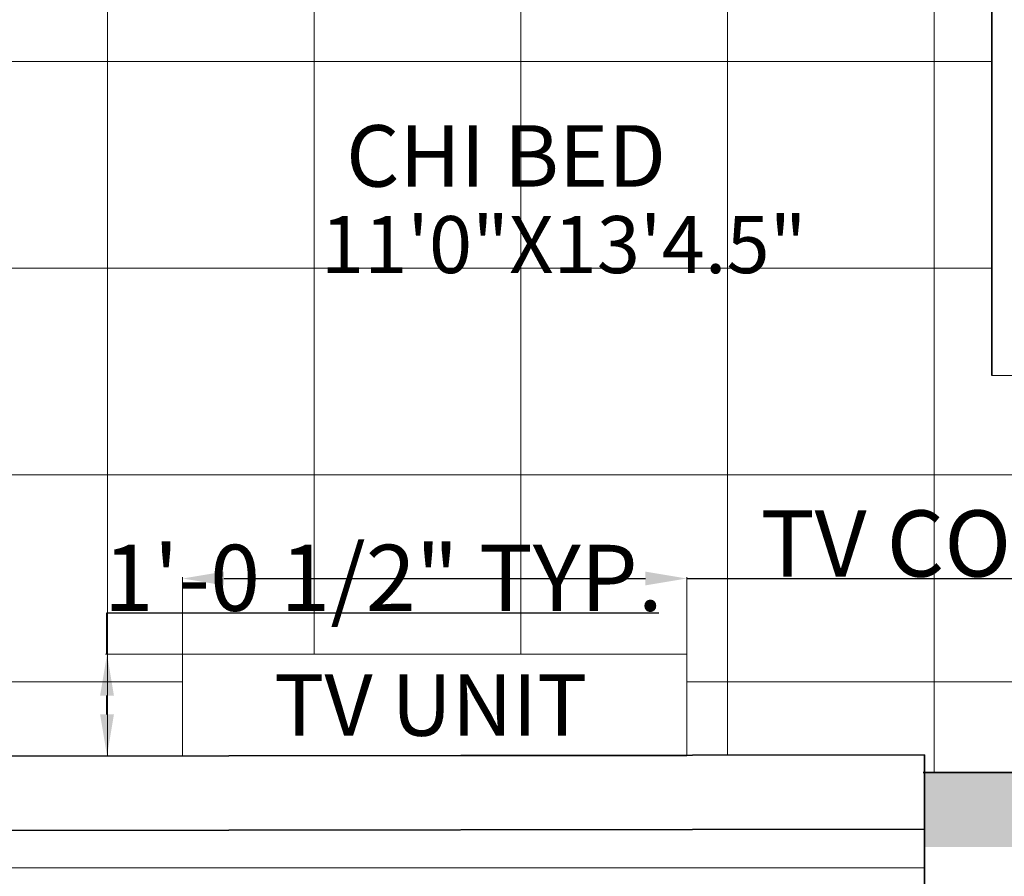
# Model space of a CAD drawing. Units: inches. Extents: x 351 to 1738, y -265 to 286.
# Tile 22 of 38: x 1127 to 1246, y -63 to 41. Entities that reach past the tile are written whole.
import ezdxf

# ---------------------------------------------------------------- set-up
doc = ezdxf.new("R2010")
doc.units = ezdxf.units.IN
doc.header["$MEASUREMENT"] = 0
for name, color, linetype, lineweight in [('A-ANNO-DIMS', 2, 'Continuous', 18), ('A-ANNO-TEXT', 7, 'Continuous', 18), ('A-AREA-IDEN', 7, 'Continuous', 18), ('A-COLS-PATT', 6, 'Continuous', 13), ('A-DOOR', 3, 'Continuous', 18), ('A-FLOR-CASE', 9, 'Continuous', 18), ('A-FLOR-PATT', 9, 'Continuous', 9), ('A-WALL', 7, 'Continuous', 35)]:
    doc.layers.add(name, color=color, linetype=linetype, lineweight=lineweight)
doc.styles.add('Annotative', font='arial.ttf')
doc.styles.get("Standard").update_dxf_attribs({"font": 'arial.ttf'})
doc.dimstyles.get("Standard").update_dxf_attribs({"dimtxt": 8, "dimasz": 5, "dimexe": 0.18, "dimexo": 0.0625, "dimgap": 0.09, "dimtad": 1, "dimtoh": 1, "dimzin": 0, "dimdsep": 46, "dimlunit": 4, "dimtxsty": 'Standard', "dimcen": 0, "dimclre": 256, "dimadec": 0, "dimazin": 0, "dimtfac": 1, "dimtofl": 0, "dimtmove": 0, "dimatfit": 3, "dimfxl": 1, "dimtolj": 1, "dimtzin": 0, "dimlwe": -1, "dimarcsym": 0})

# ---------------------------------------------------------------- blocks, each defined once
blk = doc.blocks.new('CONSOLE-TV')
blk.add_lwpolyline([(0, 0), (61, 0), (61, 12.29), (0, 12.29)], close=True)
blk = doc.blocks.new('*D42')
at = {"layer": 'A-ANNO-DIMS', "transparency": 16777216}
for p, q in [((1146.8, -35.63), (1146.8, -26.36)), ((1207.8, -35.63), (1207.8, -26.36))]:
    blk.add_line(p, q, dxfattribs=at)
at = {"layer": 'A-ANNO-DIMS', "color": 0, "lineweight": -2, "transparency": 16777216}
for p, q in [((1151.8, -26.54), (1202.8, -26.54)), ((1207.8, -26.54), (1337.09, -26.54))]:
    blk.add_line(p, q, dxfattribs=at)
at = {"layer": 'A-ANNO-DIMS', "color": 0, "transparency": 16777216}
for points in [[(1151.8, -25.71), (1151.8, -27.37), (1146.8, -26.54)], [(1202.8, -25.71), (1202.8, -27.37), (1207.8, -26.54)]]:
    blk.add_solid(points, dxfattribs=at)
at = {"layer": 'Defpoints', "color": 0, "transparency": 16777216}
for p in [(1207.8, -26.54), (1146.8, -35.69), (1207.8, -35.69)]:
    blk.add_point(p, dxfattribs=at)
at = {"layer": 'A-ANNO-DIMS', "color": 0, "transparency": 16777216, "insert": (1274.95, -22.31), "char_height": 8, "attachment_point": 5}
blk.add_mtext('\\A1;TV CONSOLE 5\'-1" TYP.', dxfattribs=at)
blk = doc.blocks.new('*D43')
at = {"layer": 'A-ANNO-DIMS', "color": 0, "lineweight": -2, "transparency": 16777216}
for p, q in [((1137.65, -35.69), (1137.65, -30.69)), ((1137.65, -30.69), (1204.4, -30.69)), ((1137.65, -42.98), (1137.65, -40.69))]:
    blk.add_line(p, q, dxfattribs=at)
at = {"layer": 'A-ANNO-DIMS', "transparency": 16777216}
for p, q in [((1146.74, -35.69), (1137.47, -35.69)), ((1146.74, -47.98), (1137.47, -47.98))]:
    blk.add_line(p, q, dxfattribs=at)
at = {"layer": 'A-ANNO-DIMS', "color": 0, "transparency": 16777216}
for points in [[(1136.82, -40.69), (1138.49, -40.69), (1137.65, -35.69)], [(1136.82, -42.98), (1138.49, -42.98), (1137.65, -47.98)]]:
    blk.add_solid(points, dxfattribs=at)
at = {"layer": 'Defpoints', "color": 0, "transparency": 16777216}
for p in [(1137.65, -35.69), (1146.8, -35.69), (1146.8, -47.98)]:
    blk.add_point(p, dxfattribs=at)
at = {"layer": 'A-ANNO-DIMS', "color": 0, "transparency": 16777216, "insert": (1171.07, -26.46), "char_height": 8, "attachment_point": 5}
blk.add_mtext('\\A1;1\'-0 1/2" TYP.', dxfattribs=at)
blk = doc.blocks.new('*D52')
at = {"layer": 'A-ANNO-DIMS', "color": 0, "lineweight": -2, "transparency": 16777216}
for p, q in [((1098.3, 46.26), (1098.3, 51.26)), ((1098.3, 51.26), (1235.28, 51.26)), ((1098.3, 15.26), (1098.3, 41.26))]:
    blk.add_line(p, q, dxfattribs=at)
at = {"layer": 'A-ANNO-DIMS', "transparency": 16777216}
for p, q in [((1103.64, 46.26), (1098.12, 46.26)), ((1103.64, 10.26), (1098.12, 10.26))]:
    blk.add_line(p, q, dxfattribs=at)
at = {"layer": 'A-ANNO-DIMS', "color": 0, "transparency": 16777216}
for points in [[(1097.47, 41.26), (1099.14, 41.26), (1098.3, 46.26)], [(1097.47, 15.26), (1099.14, 15.26), (1098.3, 10.26)]]:
    blk.add_solid(points, dxfattribs=at)
at = {"layer": 'Defpoints', "color": 0, "transparency": 16777216}
for p in [(1098.3, 46.26), (1103.7, 46.26), (1103.7, 10.26)]:
    blk.add_point(p, dxfattribs=at)
at = {"layer": 'A-ANNO-DIMS', "color": 0, "transparency": 16777216, "insert": (1166.84, 55.49), "char_height": 8, "attachment_point": 5}
blk.add_mtext('\\A1;STAIR WINDOW 3\'-0" TYP.', dxfattribs=at)

msp = doc.modelspace()

# ---------------------------------------------------------------- hatches: boundary and pattern name
at = {"layer": 'A-COLS-PATT'}
h = msp.add_hatch(color=256, dxfattribs=at)
h.dxf.hatch_style = 1
h.paths.add_polyline_path([(1112.704, 237.963), (1103.704, 237.963), (1103.704, 228.963), (1112.704, 228.963)])
h.paths.add_polyline_path([(1115.704, 237.963), (1112.704, 237.963), (1112.704, 228.963), (1115.704, 228.963)])
h.paths.add_polyline_path([(1043.704, 255.963), (1034.704, 255.963), (1034.704, 243.963), (1043.704, 243.963)])
h.paths.add_polyline_path([(1043.704, 210.963), (1034.704, 210.963), (1034.704, 198.963), (1043.704, 198.963)])
h.paths.add_polyline_path([(1043.704, -45.037), (1034.704, -45.037), (1034.704, -57.037), (1043.704, -57.037)])
h.paths.add_polyline_path([(1112.704, -45.037), (1103.704, -45.037), (1103.704, -57.037), (1112.704, -57.037)])
h.paths.add_polyline_path([(1112.704, -161.037), (1103.704, -161.037), (1103.704, -164.037), (1103.704, -173.037), (1112.704, -173.037)])
h.paths.add_polyline_path([(1043.704, -161.037), (1034.704, -161.037), (1034.704, -173.037), (1043.704, -173.037)])
h.paths.add_polyline_path([(1248.549, -164.037), (1236.549, -164.037), (1236.549, -173.037), (1248.549, -173.037)])
h.paths.add_polyline_path([(1248.549, -50), (1236.549, -50), (1236.549, -59), (1248.549, -59)])
h.paths.add_polyline_path([(1248.704, 73.463), (1244.704, 73.463), (1244.704, 64.463), (1248.704, 64.463)])
h.paths.add_polyline_path([(1244.704, 73.463), (1236.704, 73.463), (1236.704, 64.463), (1244.704, 64.463)])
h.paths.add_polyline_path([(1248.704, 237.963), (1236.704, 237.963), (1236.704, 228.963), (1248.704, 228.963)])
h.paths.add_polyline_path([(1392.204, 237.963), (1380.204, 237.963), (1380.204, 228.963), (1392.204, 228.963)])
h.paths.add_polyline_path([(1536.064, 237.963), (1524.064, 237.963), (1524.064, 228.963), (1536.064, 228.963)])
h.paths.add_polyline_path([(1536.064, 73.463), (1524.064, 73.463), (1524.064, 64.463), (1536.064, 64.463)])
h.paths.add_polyline_path([(1384.204, 73.463), (1380.204, 73.463), (1380.204, 64.463), (1384.204, 64.463)])
h.paths.add_polyline_path([(1392.064, 73.463), (1384.204, 73.463), (1384.204, 64.463), (1392.064, 64.463)])
h.paths.add_polyline_path([(1536.064, -53.037), (1524.064, -53.037), (1524.064, -57.037), (1536.064, -57.037)])
h.paths.add_polyline_path([(1536.064, -48.037), (1524.064, -48.037), (1524.064, -53.037), (1536.064, -53.037)])
h.paths.add_polyline_path([(1392.064, -48.037), (1380.064, -48.037), (1380.064, -56.5), (1380.065, -57.037), (1392.064, -57.037)])
h.paths.add_polyline_path([(1536.064, -164.037), (1524.064, -164.037), (1524.064, -173.037), (1536.064, -173.037)])
at = {"layer": 'A-FLOR-PATT', "transparency": 33554559}
h = msp.add_hatch(dxfattribs=at)
h.set_pattern_fill('ANSI37', color=256, scale=200, angle=135)
h.set_pattern_definition([(180, (1112.704, -164.037), (-2e-15, -25), []), (270, (1112.704, -164.037), (25, -5e-15), [])])
h.paths.add_polyline_path([(1380.064, 73.463), (1380.132, 148.463), (1338.064, 148.463), (1290.704, 148.463), (1290.704, 88.463), (1248.704, 88.463), (1248.704, -2.009), (1244.704, -2.009), (1244.704, 142.457), (1160.704, 142.457), (1160.704, 158.963), (1160.704, 170.137), (1160.704, 206.137), (1160.704, 228.963), (1112.704, 228.963), (1112.704, 209.963), (1112.704, 168.963), (1124.704, 168.963), (1124.704, 162.963), (1112.704, 162.963), (1112.704, 64.463), (1112.704, 60.463), (1112.704, 0.463), (1112.704, -48.026), (1146.804, -47.981), (1146.804, -35.691), (1207.804, -35.691), (1207.804, -47.902), (1236.542, -47.864), (1236.544, -50.009), (1248.5, -50.009), (1248.506, -102.915), (1248.512, -150.915), (1248.514, -164.037), (1248.549, -164.037), (1273.017, -164.037), (1273.017, -128.799), (1355.24, -128.799), (1355.24, -164.037), (1384.204, -164.037), (1384.204, -57.037), (1380.064, -57.037), (1380.064, -48.037), (1392.064, -48.037), (1392.064, -53.037), (1406.549, -53.037), (1406.549, -57.037), (1401.204, -57.037), (1401.204, -147.037), (1468.204, -147.037), (1468.204, -138.5), (1472.204, -138.5), (1472.204, -102.5), (1468.204, -102.5), (1468.204, -57.037), (1442.549, -57.037), (1442.549, -53.037), (1463.049, -53.037), (1463.049, -40.747), (1524.049, -40.747), (1524.049, -48.037), (1536.064, -48.037), (1536.064, -53.037), (1557.704, -53.037), (1557.704, 204.963), (1384.204, 204.963), (1384.204, 73.463), (1392.064, 73.463), (1392.064, 64.463), (1384.204, 64.463), (1384.204, -3.5), (1380.204, -3.537), (1380.204, 64.463), (1380.064, 64.463)])
h.paths.add_polyline_path([(1510.714, 86.458, -0.1039845), (1511.661, 85.595, 0.4704384), (1510.158, 87.614, 0.0961001)], flags=16)
h.paths.add_polyline_path([(1510.443, 100.266, 0.009798), (1504.693, 100.48, 0.0287898), (1504.6, 99.767, -0.1653311), (1505.519, 96.135, -0.1436014)], flags=16)
h.paths.add_polyline_path([(1487.201, 85.595, -0.1039845), (1488.148, 86.458, 0.0961001), (1488.704, 87.614, 0.4704384)], flags=0)
h.paths.add_polyline_path([(1495.052, 100.43), (1494.178, 100.43, -0.0264629), (1494.262, 99.774, -0.1442193)], flags=16)
h.paths.add_polyline_path([(1444.485, 86.458, -0.1039845), (1445.433, 85.595, 0.4704384), (1443.93, 87.614, 0.0961001)], flags=16)
h.paths.add_polyline_path([(1420.972, 85.595, -0.1039845), (1421.92, 86.458, 0.0961001), (1422.475, 87.614, 0.4704384)], flags=16)
h.paths.add_polyline_path([(1428.632, 100.335, 0.0010541), (1427.971, 100.309, -0.0215241), (1428.033, 99.774, -0.1143008)], flags=16)
h.paths.add_polyline_path([(1419.906, 143.708, 0.0249793), (1420.222, 157.526), (1421.573, 159.101), (1421.573, 175.369), (1391.393, 175.369), (1391.393, 200.519), (1542.294, 200.519), (1542.294, 175.369), (1512.028, 175.369, 0.0198653), (1511.521, 153.838, 0.0251335), (1512.758, 118.323, 0.0205529), (1512.942, 115.253), (1419.834, 115.253, -0.0004142), (1419.843, 124.798), (1413.059, 124.798), (1413.059, 84.437, -0.0618528), (1415.831, 80.45, -0.0930773), (1420.972, 85.595, -0.2675367), (1422.371, 84.732, 0.0851103), (1424.052, 84.616, -0.8853927), (1424.033, 84.851, -1.1258145), (1424.073, 84.366, -0.0879871), (1422.371, 84.732, -0.2675367), (1422.326, 83.089, -0.3705421), (1420.972, 85.595, 0.0930773), (1415.831, 80.45, -0.0874142), (1417.914, 73.937), (1418.941, 73.937, 0.0272504), (1418.913, 76.906, -0.1157032), (1421.051, 73.937), (1445.354, 73.937, -0.1157032), (1447.492, 76.906, 0.0272504), (1447.464, 73.937), (1448.491, 73.937, -0.0874142), (1450.574, 80.45, 0.0930773), (1445.433, 85.595, -0.3705421), (1444.079, 83.089, -0.2675367), (1444.034, 84.732, -0.0879871), (1442.332, 84.366, -1.1258145), (1442.372, 84.851, -2.0327363), (1442.364, 84.368, 0.0863779), (1444.034, 84.732, -0.2675367), (1445.433, 85.595, -0.0930773), (1450.574, 80.45, -0.2577317), (1466.483, 90.927, -0.4786702), (1468.832, 91.907, -0.4786702), (1471.18, 90.927, -0.26264), (1483.053, 81.78, -0.0718662), (1487.201, 85.595, -0.2675367), (1488.6, 84.732, 0.0851103), (1490.28, 84.616, -0.8853927), (1490.262, 84.851, -1.1258145), (1490.301, 84.366, -0.0879871), (1488.6, 84.732, -0.2675367), (1488.554, 83.089, -0.3705421), (1487.201, 85.595, 0.0718662), (1483.053, 81.78, -0.1320648), (1484.143, 73.937), (1485.169, 73.937, 0.0272504), (1485.142, 76.906, -0.1157032), (1487.28, 73.937), (1511.582, 73.937, -0.1157032), (1513.72, 76.906, 0.0272504), (1513.693, 73.937), (1514.719, 73.937, -0.0874142), (1516.802, 80.45, 0.0930773), (1511.661, 85.595, -0.3705421), (1510.308, 83.089, -0.2675367), (1510.262, 84.732, -0.0879871), (1508.561, 84.366, -1.1258145), (1508.601, 84.851, -2.0327363), (1508.592, 84.368, 0.0863779), (1510.262, 84.732, -0.2675367), (1511.661, 85.595, -0.0930773), (1516.802, 80.45, -0.0618528), (1519.575, 84.437), (1519.575, 73.937), (1413.059, 73.937), (1413.059, 124.798), (1419.843, 124.798, -0.0008205)], flags=16)
h.paths.add_polyline_path([(1220.149, 54.133, -0.1039845), (1220.869, 53.476, 0.4704384), (1219.727, 55.011, 0.0961001)], flags=16)
h.paths.add_polyline_path([(1219.944, 64.626, 0.009798), (1215.574, 64.789, 0.0287898), (1215.503, 64.247, -0.1653311), (1216.201, 61.487, -0.1436014)], flags=16)
h.paths.add_polyline_path([(1209.779, 64.449, 0.0974459), (1209.339, 64.751), (1208.247, 64.751, 0.1273905), (1207.7, 64.326, 0.1715858), (1206.95, 61.475, -0.1588542), (1207.636, 59.45, 0.0158984), (1207.795, 59.218, 0.0615457), (1208.598, 59.616, 0.1754158), (1208.638, 60.099, -0.2847793), (1209.348, 62.472, 0.3262165)], flags=16)
h.paths.add_polyline_path([(1169.818, 54.133, -0.1039845), (1170.538, 53.476, 0.4704384), (1169.396, 55.011, 0.0961001)], flags=16)
h.paths.add_polyline_path([(1159.017, 62.472, 0.2847642), (1158.307, 60.099, -0.1754332), (1158.267, 59.616, 0.3929302), (1159.448, 64.449, -0.3262298)], flags=16)
h.paths.add_polyline_path([(1156.342, 58.239, -0.1783213), (1154.011, 55.31, -0.1747359), (1154.722, 55.233, -0.2008015), (1156.27, 56.086, 0.1269899), (1157.283, 58.991, -0.0912053)], flags=16)
h.paths.add_polyline_path([(1156.624, 61.413, 0.1572752), (1157.316, 64.247, 0.1696217)], flags=16)
h.paths.add_polyline_path([(1152.67, 54.133, -0.0961001), (1151.95, 53.476, 0.0640762), (1154.465, 54.384, 0.1990158)], flags=16)
h.paths.add_polyline_path([(1202.281, 53.476, -0.1039845), (1203, 54.133, 0.0961001), (1203.423, 55.011, 0.4704384)], flags=0)
h.paths.add_polyline_path([(1151.139, 97.64, 0.0249793), (1151.379, 108.141), (1152.406, 109.338), (1152.406, 121.701), (1129.47, 121.701), (1129.47, 140.814), (1244.149, 140.814), (1244.149, 121.701), (1221.148, 121.701, 0.0198653), (1220.763, 105.338, 0.0251335), (1221.703, 78.349, 0.0205529), (1221.843, 76.016), (1151.078, 76.016, -0.1287433), (1148.786, 65.037, 0.5393525), (1150.327, 64.171, -0.027594), (1163.481, 64.751, 0.0976954), (1163.04, 64.449, 0.3262165), (1163.471, 62.472, -0.2847765), (1164.181, 60.099, -0.1947567), (1165.846, 61.443, -0.1554021), (1165.172, 64.247, -0.1660224), (1165.869, 61.475, -0.1770142), (1167.852, 62.77, -0.4482027), (1169.974, 60.807, -0.3934987), (1167.679, 57.86, -0.8955483), (1168.438, 54.524, -0.3557668), (1166.218, 56.086, -0.066024), (1165.505, 57.539), (1165.251, 56.243, -0.3717324), (1164.02, 59.758, -0.3736141), (1163.04, 64.449, -0.0976954), (1163.481, 64.751, 0.0213538), (1153.294, 64.429, -0.1341826), (1156.695, 61.368, 0.1868727), (1154.636, 62.77, 0.4482027), (1152.514, 60.807, 0.4037263), (1154.905, 57.846, 0.7112192), (1153.334, 55, 0.5315397), (1151.95, 53.476, -0.2675367), (1153.013, 52.821, 0.0851103), (1154.29, 52.732, -0.8853927), (1154.276, 52.911, -1.1258145), (1154.306, 52.543, -0.0879871), (1153.013, 52.821, -0.2675367), (1152.978, 51.572, -0.3705421), (1151.95, 53.476, 0.0930773), (1148.043, 49.566, -0.0874142), (1149.626, 44.617), (1150.406, 44.617, 0.0272504), (1150.385, 46.873, -0.1157032), (1152.01, 44.617), (1170.478, 44.617, -0.1157032), (1172.103, 46.873, 0.0272504), (1172.082, 44.617), (1172.862, 44.617, -0.0874142), (1174.445, 49.566, 0.0930773), (1170.538, 53.476, -0.3705421), (1169.51, 51.572, -0.2675367), (1169.475, 52.821, -0.0879871), (1168.182, 52.543, -1.1258145), (1168.212, 52.911, -2.0327363), (1168.206, 52.544, 0.0863779), (1169.475, 52.821, -0.2675367), (1170.538, 53.476, -0.0930773), (1174.445, 49.566, -0.2577317), (1186.536, 57.528, -0.4786702), (1188.321, 58.273, -0.4786702), (1190.106, 57.528, -0.26264), (1199.128, 50.577, -0.0718662), (1202.281, 53.476, -0.2675367), (1203.344, 52.821, 0.0851103), (1204.621, 52.732, -0.8853927), (1204.607, 52.911, -1.1258145), (1204.637, 52.543, -0.0879871), (1203.344, 52.821, -0.2675367), (1203.309, 51.572, -0.3705421), (1202.281, 53.476, 0.0718662), (1199.128, 50.577, -0.1320648), (1199.957, 44.617), (1200.737, 44.617, 0.0272504), (1200.716, 46.873, -0.1157032), (1202.341, 44.617), (1220.809, 44.617, -0.1157032), (1222.434, 46.873, 0.0272504), (1222.413, 44.617), (1223.193, 44.617, -0.0874142), (1224.776, 49.566, 0.0930773), (1220.869, 53.476, -0.3705421), (1219.841, 51.572, -0.2675367), (1219.806, 52.821, -0.0879871), (1218.513, 52.543, -1.1258145), (1218.543, 52.911, -2.0327363), (1218.537, 52.544, 0.0863779), (1219.806, 52.821, -0.2675367), (1220.869, 53.476, -0.0930773), (1224.776, 49.566, -0.0618528), (1226.883, 52.597), (1226.883, 44.617), (1145.936, 44.617), (1145.936, 83.269), (1151.091, 83.269, -0.0008205)], flags=16)
h.paths.add_polyline_path([(1218.01, 57.86, -0.8955483), (1218.769, 54.524, -0.3557668), (1216.549, 56.086, -0.066024), (1215.836, 57.539), (1215.582, 56.243, -0.3717324), (1214.351, 59.758, -0.3736141), (1213.371, 64.449, 0.3262165), (1213.802, 62.472, -0.2847765), (1214.512, 60.099, -0.1947567), (1216.177, 61.443, -0.1799907), (1218.183, 62.77, -0.4482027), (1220.305, 60.807, -0.3934987)], flags=16)
h.paths.add_polyline_path([(1424.735, 91.363, -0.3934987), (1421.715, 95.241, -0.4482027), (1424.507, 97.824, -0.1799907), (1427.147, 96.077, -0.1947567), (1429.338, 94.309, -0.2847765), (1430.272, 97.432, 0.3262165), (1430.839, 100.034, -0.3736141), (1429.55, 93.861, -0.3717324), (1427.929, 89.235), (1427.596, 90.941, -0.066024), (1426.657, 89.029, -0.3557668), (1423.736, 86.973, -0.8955483)], flags=16)
h.paths.add_polyline_path([(1238.033, 131.257, -1), (1227.329, 131.257, -1)], flags=0)
h.paths.add_polyline_path([(1235.357, 131.257, -1), (1230.005, 131.257, -1)], flags=0)
h.paths.add_polyline_path([(1214.039, 54.243, 0.1543819), (1214.38, 53.992, 0.3589549), (1213.613, 54.016, 0.6039484), (1214.379, 53.657, 0.3713191), (1213.968, 52.872, 0.1879935), (1214.312, 52.809, -0.592455), (1213.953, 52.967, -0.2942791), (1214.083, 53.691, -1.3001871), (1213.881, 54.134, -0.2837621), (1214.469, 53.896, 1.1509396)], flags=16)
h.paths.add_polyline_path([(1212.091, 56.286, -0.4084338), (1211.337, 56.445, -0.0362594), (1211.098, 56.848, -0.2360976), (1211.59, 56.63, 0.0353445), (1211.835, 56.543, -0.4752408), (1212.091, 56.286, -0.4752408), (1212.438, 56.182, 0.0353445), (1212.631, 56.007, -0.2360976), (1213.056, 55.676, -0.0362594), (1212.588, 55.697, -0.4084338)], flags=16)
h.paths.add_polyline_path([(1211.469, 50.297, 0.296043), (1210.47, 50.527, 0.310883), (1211.931, 50.148, 0.0212546)], flags=16)
h.paths.add_polyline_path([(1213.739, 51.818, -0.0362594), (1213.271, 51.838, -0.4084337), (1212.774, 52.427, -0.0947856), (1212.293, 50.703, 1.1504738), (1212.911, 50.232, 0.1662877), (1213.265, 50.68, -0.0252543), (1212.603, 50.13, 1.0879317), (1212.471, 49.407, 0.1662877), (1213.02, 49.251, -0.016128), (1212.567, 49.563, -0.286859), (1212.217, 49.638, 0.0221563), (1212.046, 50.055, -0.6461302), (1212.185, 50.498, 0.0884116), (1212.732, 52.077, -1.1860374), (1213.121, 52.323, 0.0353445), (1213.314, 52.148, -0.2360976)], flags=16)
h.paths.add_polyline_path([(1212.094, 50.342, -0.0485241), (1211.54, 49.605, -1.1038339), (1211.397, 48.738, -0.7855147), (1211.683, 48.254, -0.3920429), (1210.948, 48.525, -0.3928194), (1210.561, 47.995, -0.592455), (1210.201, 48.153, -0.2942791), (1210.331, 48.877, -0.7041716), (1210.316, 49.592, -0.6793441), (1210.729, 50.112, 0.5636764)], flags=16)
h.paths.add_polyline_path([(1211.274, 49.829, -0.1398258), (1210.745, 49.859, -0.2178785), (1210.948, 49.509, -0.4985724)], flags=0)
h.paths.add_polyline_path([(1433.426, 81.49, -0.181571), (1434.245, 81.788, -0.0080665), (1433.726, 82.205, 0.0455784), (1432.755, 81.242, 0.1790113)], flags=16)
h.paths.add_polyline_path([(1434.146, 81.009, -0.1324418), (1433.645, 80.771, 0.2590893), (1433.234, 80.471, -0.1802109), (1433.392, 80.805, -0.1699398), (1432.758, 81.109, 0.0326525), (1433.273, 80.474, -0.4933627), (1434.046, 80.146, -0.3904966)], flags=16)
h.paths.add_polyline_path([(1434.83, 80.047, -0.9475376), (1435.294, 79.576, -0.2991282), (1434.625, 79.404, -0.2704392), (1435.01, 78.591, -0.592455), (1434.537, 78.382, -0.3928194), (1434.027, 79.08, -0.3920429), (1433.06, 78.723, -0.3520423), (1433.003, 79.197, -0.1972159), (1433.75, 79.734, -0.7136405), (1434.447, 79.939, -0.2147903), (1434.819, 80.475, 0.4088333), (1435.075, 80.803, -0.2261519)], flags=16)
h.paths.add_polyline_path([(1432.67, 81.217, -0.4542182), (1431.897, 79.923, -0.4144105), (1431.301, 80.035, 0.0161291), (1431.897, 80.445, 0.2795702), (1432.073, 80.871, -0.2895037), (1431.103, 81.321, -0.4144105), (1430.978, 81.915, 0.0161296), (1431.586, 81.521, 0.341293), (1432.125, 81.583, -0.8131856)], flags=16)
h.paths.add_polyline_path([(1429.893, 86.381, -0.9475376), (1430.358, 85.91, -0.1731062), (1429.984, 85.712, -0.0388172), (1431.625, 84.214, -0.0879005), (1432.097, 88.549, -0.0497684), (1431.254, 88.49, -0.2360976), (1431.814, 88.925, 0.0353445), (1432.067, 89.155, -0.4752408), (1432.524, 89.291, -0.4752408), (1432.86, 89.63, 0.0353445), (1433.182, 89.744, -0.2360976), (1433.83, 90.032, -0.0362594), (1433.516, 89.502, -0.4084338), (1432.524, 89.291, -0.3124239), (1432.106, 88.58, 0.0885594), (1431.625, 84.214, -0.4084337), (1430.971, 83.439, -0.0362594), (1430.355, 83.412, -0.2360976), (1430.914, 83.847, 0.0353445), (1431.168, 84.078, -0.4752408), (1431.625, 84.214, 0.0388172), (1429.984, 85.712, -0.3217316), (1429.333, 86.048, -0.32743), (1429.883, 86.809, 0.4088333), (1430.138, 87.138, -0.2261519)], flags=16)
h.paths.add_polyline_path([(1211.206, 58.616, -0.9997836), (1211.336, 59.323, -0.6149935)], flags=16)
h.paths.add_polyline_path([(1210.288, 49.429, 0.1543819), (1210.629, 49.178, 0.3589549), (1209.861, 49.202, 0.6039484), (1210.627, 48.843, -0.5348247), (1210.806, 49.295, 0.7483464)], flags=16)
h.paths.add_polyline_path([(1209.589, 51.828, -0.0087906), (1209.775, 51.753, 0.1122315), (1209.466, 52.019, 1.4188509), (1209.014, 51.708, -0.4587257), (1208.651, 51.073, -0.592455), (1208.291, 51.232, -0.2942791), (1208.421, 51.955, -1.3001871), (1208.219, 52.398, -0.2260052), (1208.719, 52.257, -0.4755189), (1209.158, 52.369, -1.4554994), (1209.603, 52.664, 0.4213049), (1209.191, 52.262, -0.5912116), (1208.979, 51.796, 0.4973986), (1209.773, 51.333, 0.6493116)], flags=16)
h.paths.add_polyline_path([(1208.029, 52.041, 0.5446671), (1208.832, 52.045, 0.220132)], flags=0)
h.paths.add_polyline_path([(1210.438, 51.425, -0.2041997), (1210.277, 52.018, 0.2708262), (1209.915, 52.897, 0.3241145)], flags=0)
h.paths.add_polyline_path([(1209.668, 52.407, -0.60139), (1208.99, 52.221, -0.3949159), (1208.248, 52.83, -0.8367916), (1208.651, 53.017, -0.3384876), (1209.039, 52.571, 0.1941379), (1209.191, 52.262, 0.4139945), (1209.712, 52.475, 0.5177103), (1210.503, 51.416, 0.401922), (1209.493, 50.93, 0.2063956), (1209.516, 50.165, -0.3194629), (1210.417, 51.418, -0.466635)], flags=16)
h.paths.add_polyline_path([(1206.601, 56.086, -0.3557668), (1204.381, 54.524, -0.9211983), (1205.236, 57.846, 0.2065693), (1207.614, 58.991, -0.1269899)], flags=16)
h.paths.add_polyline_path([(1435.487, 82.816, 0.5277653), (1436.615, 83.361, 0.5085402), (1437.05, 82.433, 0.592455), (1437.524, 82.641, 0.3312448), (1436.963, 83.548, 0.3878632), (1437.808, 83.626, 0.5929544), (1437.618, 84.176, 0.2260158), (1436.961, 83.99, 0.3182053), (1437.588, 84.854, 0.6893744), (1437.05, 84.991, 0.3357648), (1436.539, 84.41, -0.1569934), (1436.404, 84.065, -0.4346112), (1436.961, 83.99, -0.2147903), (1437.333, 84.526, 0.4088333), (1437.588, 84.854, -0.2261519), (1437.343, 84.097, -0.9475376), (1437.808, 83.626, -0.2991282), (1437.139, 83.455, -0.2704392), (1437.524, 82.641, -0.592455), (1437.05, 82.433, -0.3928194), (1436.541, 83.13, -0.4396601), (1435.475, 82.794, -0.174614), (1435.942, 82.244, -0.2063956), (1435.912, 81.237, -0.2708262), (1435.125, 82.208, 0.2079765), (1434.686, 82.904, -0.1964955)], flags=16)
h.paths.add_polyline_path([(1435.386, 84.832, 0.270811), (1434.91, 83.676, -0.2042174), (1434.699, 82.895, 0.3241145)], flags=0)
h.paths.add_polyline_path([(1435.68, 84.18, -0.2176564), (1435.554, 83.304, -0.1767045), (1436.236, 83.778, -0.3730364)], flags=0)
h.paths.add_polyline_path([(1435.566, 100.034, 0.3262165), (1436.133, 97.432, -0.2847765), (1437.067, 94.309, -0.1947567), (1439.258, 96.077, -0.1554021), (1438.371, 99.767, -0.1660224), (1439.289, 96.12, -0.1770142), (1441.897, 97.824, -0.4482027), (1444.69, 95.241, -0.3934987), (1441.67, 91.363, -0.8955483), (1442.669, 86.973, -0.3557668), (1439.748, 89.029, -0.066024), (1438.809, 90.941), (1438.476, 89.235, -0.3717324), (1436.855, 93.861, -0.3736141)], flags=16)
h.paths.add_polyline_path([(1191.252, 49.507, -0.2740221), (1190.658, 48.409, 0.2675367), (1191.311, 47.344, 0.3705421)], flags=0)
h.paths.add_polyline_path([(1190.301, 49.717, 0.1990158), (1188.619, 49.04, 0.0640762), (1191.252, 49.507, -0.0961001)], flags=0)
h.paths.add_polyline_path([(1189.518, 47.857, 1.1258145), (1189.676, 47.523, 2.0446052)], flags=0)
h.paths.add_polyline_path([(1464.974, 80.372, 0.2740221), (1465.756, 78.927, -0.0830131)], flags=0)
h.paths.add_polyline_path([(1464.974, 80.372, 0.3705421), (1464.897, 77.525, 0.5763244)], flags=0)
h.paths.add_polyline_path([(1464.974, 80.372, -0.4704384), (1467.284, 81.372, -0.0961001), (1466.226, 80.648, -0.1990158), (1468.439, 79.757, -0.0640762)], flags=0)
h.paths.add_polyline_path([(1189.511, 56.43, -0.2594668), (1188.321, 56.391, -0.2594668), (1187.13, 56.43, 0.0851103), (1188.193, 55.716, -0.8853927), (1188.27, 55.878, -1.1960133), (1188.355, 55.442, 0.1014587)], flags=0)
h.paths.add_polyline_path([(1188.321, 57.596, 0.0780722), (1187.678, 57.24, 0.0155503), (1188.321, 57.136, 0.0155503), (1188.964, 57.24, 0.0780722)], flags=0)
h.paths.add_polyline_path([(1190.164, 55.365, -0.5763244), (1190.106, 57.528, -0.1982945), (1188.321, 58.319, -0.1982945), (1186.536, 57.528, -0.5763244), (1186.477, 55.365, -0.3705421), (1186.536, 57.528, 0.1982945), (1188.321, 58.319, 0.1982945), (1190.106, 57.528, -0.3705421)], flags=0)
h.paths.add_polyline_path([(1188.372, 55.878, 1.1258145), (1188.529, 55.544, 2.0446052)], flags=0)
h.paths.add_polyline_path([(1186.341, 49.717, -0.0961001), (1185.389, 49.507, 0.0640762), (1188.022, 49.04, 0.1990158)], flags=0)
h.paths.add_polyline_path([(1185.389, 49.507, -0.2675367), (1185.984, 48.409, 0.0851103), (1187.046, 47.695, -0.8853927), (1187.123, 47.857, -1.1258145), (1186.966, 47.523, -0.0879871), (1185.984, 48.409, -0.2675367), (1185.331, 47.344, -0.3705421)], flags=0)
h.paths.add_polyline_path([(1399.441, 187.944, -1), (1413.525, 187.944, -1)], flags=0)
h.paths.add_polyline_path([(1402.962, 187.944, -1), (1410.004, 187.944, -1)], flags=0)
h.paths.add_polyline_path([(1357.663, -72.245), (1377.272, -72.245), (1377.272, -91.854), (1357.663, -91.854)], flags=16)
h.paths.add_polyline_path([(1467.256, 78.201, -1.1258145), (1467.049, 77.761, -2.0446052)], flags=0)
h.paths.add_polyline_path([(1468.822, 88.714, 0.9411249), (1469.106, 88.316, 1.1371523), (1468.765, 88.755, 0.890986), (1468.99, 88.245, 0.0948283), (1470.398, 89.481, -0.2675367), (1471.18, 90.927, -0.0281232), (1469.678, 90.547, -0.0287737), (1469.948, 90.311, -0.0203267), (1468.832, 90.41, -0.0203267), (1467.716, 90.311, -0.0287737), (1467.986, 90.547, -0.0281232), (1466.483, 90.927, -0.2675367), (1467.265, 89.481, 0.0851103), (1468.663, 88.542, -1.2023159)], flags=0)
h.paths.add_polyline_path([(1178.25, 124.523, -0.1199286), (1165.65, 124.145, -0.1073492), (1159.133, 124.446, -0.1028906), (1159.132, 130.465, -0.0748968), (1158.993, 137.956, 0.002027), (1167.844, 137.479, -0.07553), (1180.337, 137.666, -0.0758613), (1186.502, 137.688, -0.1409896), (1186.272, 130.046, -0.0954805), (1186.729, 124.748, -0.10603)], flags=0)
h.paths.add_polyline_path([(1469.225, 79.757, -0.1990158), (1471.437, 80.648, -0.0961001), (1470.379, 81.372, -0.4704384), (1472.689, 80.372, -0.3705421), (1472.766, 77.525, -0.2675367), (1471.907, 78.927, -0.0879863), (1470.615, 77.761, -1.1258491), (1470.408, 78.201, -2.0327363), (1470.642, 77.778, 0.0863779), (1471.907, 78.927, -0.2675367), (1472.689, 80.372, -0.0640762)], flags=0)
h.paths.add_polyline_path([(1430.423, 186.902, -0.0748968), (1430.24, 196.758, 0.002027), (1441.887, 196.131, -0.07553), (1458.326, 196.377, -0.0758613), (1466.438, 196.406, -0.1409896), (1466.136, 186.35, -0.0954805), (1466.737, 179.378, -0.10603), (1455.58, 179.082, -0.1199286), (1439, 178.585, -0.1073492), (1430.425, 178.981, -0.1028906)], flags=0)
h.paths.add_polyline_path([(1162.258, 49.939, 0.3357645), (1161.87, 49.497, -0.1569936), (1161.767, 49.235, -0.4346112), (1162.19, 49.178, -0.2147903), (1162.473, 49.585, 1.5291948)], flags=16)
h.paths.add_polyline_path([(1161.683, 49.021, 0.5815181), (1161.268, 49.583, 0.5927609)], flags=16)
h.paths.add_polyline_path([(1162.602, 48.058, 0.3713191), (1162.192, 48.843, 0.4345332), (1162.88, 48.962, 0.1850806), (1162.197, 48.926, 1.1218369)], flags=16)
h.paths.add_polyline_path([(1161.443, 48.941, -1.3071038), (1161.495, 48.571, -0.2177521), (1161.136, 48.254, 0.6973029), (1161.871, 49.048, 0.1215141)], flags=16)
h.paths.add_polyline_path([(1162.531, 49.429, -0.2070837), (1162.05, 49.146, -0.9920299)], flags=16)
h.paths.add_polyline_path([(1161.304, 49.578, -0.7196675), (1161.513, 50.079, -0.1304275), (1160.836, 50.168, 0.0395926)], flags=0)
h.paths.add_polyline_path([(1162.036, 50.584, -0.0080665), (1161.642, 50.9, 0.0293675), (1161.35, 50.297, -0.2057884)], flags=16)
h.paths.add_polyline_path([(1162.882, 51.392, -0.1247327), (1162.763, 51.828, -0.1011907), (1162.399, 51.438, -0.153425)], flags=0)
h.paths.add_polyline_path([(1164.235, 51.85, -0.3091075), (1164.513, 51.136, -0.6271245), (1163.781, 51.603, -0.6859091), (1162.777, 51.219, -0.2332851), (1163.303, 50.165, -0.2708262), (1162.705, 50.903, 0.2041997), (1162.381, 51.425, 0.204182), (1162.542, 52.018, -0.2708414), (1162.903, 52.897, -0.1272607), (1163.219, 52.529, -1.1686811), (1163.781, 52.587, -0.3291117), (1164.168, 53.017, -0.8367917), (1164.571, 52.83, -0.1933406), (1164.391, 52.338, -0.9475376), (1164.744, 51.981, -0.2991282)], flags=16)
h.paths.add_polyline_path([(1163.598, 51.937, -1.2629561), (1163.236, 51.831, 0.0125754), (1162.971, 51.721, 0.2306566), (1163.151, 52.407, -0.1648982), (1163.178, 52.661, -0.4493201), (1163.628, 52.262, -0.721477), (1164.154, 52.088, -0.8499982)], flags=0)
h.paths.add_polyline_path([(1161.613, 58.616, -0.9804131), (1161.525, 59.049, -2.9089348)], flags=16)
h.paths.add_polyline_path([(1160.252, 49.166, -0.4144105), (1159.799, 49.251, 0.0161291), (1160.252, 49.563, 0.2795702), (1160.386, 49.887, -0.2895037), (1159.649, 50.229, -0.4144105), (1159.554, 50.68, 0.0161296), (1160.015, 50.381, 0.6178854), (1160.526, 50.703, -0.0947856), (1160.045, 52.427, -0.1404436), (1159.682, 52.042, -0.0578559), (1159.3, 51.872, 0.5448433), (1160.046, 52.419, -0.0881216), (1160.404, 55.721, -0.0497684), (1159.763, 55.676, -0.2360976), (1160.188, 56.007, 0.0353445), (1160.381, 56.182, -0.4752408), (1160.728, 56.286, -0.4752408), (1160.984, 56.543, 0.0353445), (1161.229, 56.63, -0.2360976), (1161.721, 56.848, -0.0362594), (1161.482, 56.445, -0.4084338), (1160.728, 56.286, -0.3124239), (1160.411, 55.745, 0.0885594), (1160.045, 52.427, 0.1070813), (1160.634, 50.498, -0.4947977), (1160.839, 50.149, -0.4542182)], flags=16)
h.paths.add_polyline_path([(1160.666, 49.808, -2.0765276), (1160.828, 50.172, 0.0195861)], flags=0)
h.paths.add_polyline_path([(1158.439, 53.992, 0.1543819), (1158.78, 54.243, 0.7483463), (1158.262, 54.109, -0.3382251), (1158.492, 53.839, -0.1708158), (1159.124, 53.779, 0.4957286), (1158.938, 54.134, 0.2260157)], flags=16)
h.paths.add_polyline_path([(1160.045, 52.427, 0.0388172), (1158.798, 53.565, -0.1198178), (1158.574, 53.586, -0.3091075), (1158.851, 52.872, -0.1879935), (1158.506, 52.809, 0.592455), (1158.866, 52.967, 0.3312448), (1158.44, 53.657, 0.2012451), (1158.798, 53.565, -0.034023), (1159.901, 52.578, -0.0442527), (1159.698, 52.323, -0.4752408)], flags=16)
h.paths.add_polyline_path([(1336.926, -95.392), (1336.926, -117.945), (1291.82, -117.945), (1291.82, -95.392)], flags=16)
h.paths.add_polyline_path([(1357.535, -97.244), (1357.726, -96.697, 0.0348443)], flags=16)
h.paths.add_polyline_path([(1376.693, -96.478), (1377.301, -96.5, 0.0314968), (1375.907, -96.424), (1357.726, -96.424)], flags=16)
h.paths.add_polyline_path([(1379.403, -119.667, 0.0267056), (1380.043, -119.439, -0.0152991)], flags=16)
h.paths.add_polyline_path([(1357.726, -120.202), (1357.821, -120.202), (1357.821, -120.201)], flags=16)
h.paths.add_polyline_path([(1354.171, -104.592), (1354.469, -98.672, 0.0111377)], flags=16)
h.paths.add_polyline_path([(1355.058, -119.136), (1354.578, -118.539, 0.1431635)], flags=16)
h.paths.add_polyline_path([(1378.851, -96.821), (1378.85, -96.82), (1378.85, -96.82, -0.0496798), (1380.055, -97.191), (1378.85, -96.82, 0.1500541), (1375.135, -97.188), (1375.136, -119.44, -0.0099698), (1374.747, -116.649), (1357.726, -116.649, 0.1693849), (1357.535, -119.382), (1357.535, -119.382), (1357.535, -119.382, 0.0348176), (1357.726, -119.928), (1357.726, -119.928), (1357.726, -119.929, -0.0348772), (1357.535, -119.382), (1355.507, -119.382), (1355.317, -119.278), (1357.535, -119.382, -0.1693939), (1357.726, -116.649, -0.0391513), (1374.686, -116.113, -0.0020149), (1374.625, -115.546, 0.1153223), (1369.915, -115.474, 0.0609215), (1369.922, -101.154, 0.1151459), (1374.625, -101.079, -0.0020164), (1374.686, -100.513, -0.0391511), (1357.726, -99.977), (1374.747, -99.977, -0.0099633), (1375.135, -97.188), (1375.135, -97.188, -0.1501081)], flags=16)
h.paths.add_polyline_path([(1490.963, 91.363, -0.3934987), (1487.944, 95.241, -0.4482027), (1490.736, 97.824, -0.1799907), (1493.376, 96.077, -0.1947567), (1495.567, 94.309, -0.2847765), (1496.501, 97.432, 0.3262165), (1497.068, 100.034, -0.3736141), (1495.778, 93.861, -0.3717324), (1494.158, 89.235), (1493.824, 90.941, -0.066024), (1492.886, 89.029, -0.3557668), (1489.964, 86.973, -0.8955483)], flags=16)
h.paths.add_polyline_path([(1354.86, -97.658), (1355.316, -97.348, 0.1019112)], flags=16)
h.paths.add_polyline_path([(1497.063, 83.327, 0.1767244), (1496.37, 83.785, -0.4051388), (1496.016, 83.384, 0.4973986), (1497.06, 82.774, 0.6493116), (1496.818, 83.426, -0.0087906)], flags=16)
h.paths.add_polyline_path([(1496.339, 83.783, 0.5927609), (1496.886, 84.522, 0.5815181)], flags=16)
h.paths.add_polyline_path([(1495.11, 82.641, 0.592455), (1495.583, 82.433, 0.6769152), (1495.805, 83.59, 0.3756693)], flags=16)
h.paths.add_polyline_path([(1495.015, 84.176, -0.145057), (1495.301, 84.526, -0.4088333), (1495.045, 84.854, 0.2206292), (1495.381, 84.152, -0.199594), (1495.851, 83.764, -0.5240172), (1494.826, 83.626, -0.5929976)], flags=16)
h.paths.add_polyline_path([(1501.655, 81.915, -0.0161291), (1501.048, 81.521, -0.3927187), (1500.462, 81.37, -0.2106699), (1500.607, 81.142, 0.3066994)], flags=16)
h.paths.add_polyline_path([(1500.11, 89.291, -0.4084338), (1499.118, 89.502, -0.0362594), (1498.803, 90.032, -0.2360976), (1499.451, 89.744, 0.0353445), (1499.774, 89.63, -0.4752408), (1500.11, 89.291, -0.4752408), (1500.567, 89.155, 0.0353445), (1500.82, 88.925, -0.2360976), (1501.379, 88.49, -0.0362594), (1500.763, 88.516, -0.4084338)], flags=16)
h.paths.add_polyline_path([(1498.908, 82.205, -0.0513217), (1500.013, 81.134, -0.5879306), (1500.234, 81.676, 0.1070813), (1501.009, 84.214, -0.03529)], flags=16)
h.paths.add_polyline_path([(1496.93, 83.875, -0.2063956), (1497.247, 84.832, -0.2708262), (1497.724, 83.676, 0.2079765), (1497.944, 82.884, -0.3814554)], flags=16)
h.paths.add_polyline_path([(1496.721, 81.237, 0.2708125), (1497.509, 82.208, -0.2042157), (1497.935, 82.895, 0.3241145)], flags=16)
h.paths.add_polyline_path([(1497.529, 80.125, -0.145057), (1497.814, 80.475, -0.703182), (1498.282, 81.178, -0.1229248), (1497.977, 81.714, -0.2708368), (1499.207, 81.49, 0.2079641), (1499.993, 81.248, -0.2651454), (1499.278, 80.472, 0.3819006), (1498.808, 79.947, -0.3059049), (1498.848, 79.519, 0.4994816), (1498.574, 79.217, -0.4587257), (1498.097, 78.382, -0.592455), (1497.624, 78.591, -0.2704392), (1498.009, 79.404, -0.299116), (1497.34, 79.576, -0.5930157)], flags=16)
h.paths.add_polyline_path([(1500.736, 79.923, 0.4144105), (1501.333, 80.035, -0.3216484), (1500.192, 80.765, 0.0198856), (1499.976, 81.251, 0.4653307)], flags=16)
h.paths.add_polyline_path([(1501.009, 84.214, -0.0388172), (1502.649, 85.712, -0.1730946), (1502.276, 85.91, -0.5930157), (1502.465, 86.46, -0.145057), (1502.751, 86.809, -0.4088333), (1502.495, 87.138, 0.2206292), (1502.831, 86.436, -0.199594), (1503.301, 86.048, -0.3217316), (1502.649, 85.712, 0.0388172), (1501.009, 84.214, 0.1224486), (1501.412, 83.755, 0.4754908), (1501.335, 84.226, 0.055822), (1501.719, 83.847, -0.2360976), (1502.278, 83.412, -0.0362594), (1501.663, 83.439, -0.4084338)], flags=16)
h.paths.add_polyline_path([(1501.794, 100.034, 0.3262165), (1502.362, 97.432, -0.2847765), (1503.295, 94.309, -0.1947567), (1505.486, 96.077, -0.1799907), (1508.126, 97.824, -0.4482027), (1510.918, 95.241, -0.3934987), (1507.899, 91.363, -0.8955483), (1508.898, 86.973, -0.3557668), (1505.976, 89.029, -0.066024), (1505.038, 90.941), (1504.704, 89.235, -0.3717324), (1503.084, 93.861, -0.3736141)], flags=16)
h.paths.add_polyline_path([(1146.29, 131.257, -1), (1135.587, 131.257, -1)], flags=0)
h.paths.add_polyline_path([(1143.614, 131.257, -1), (1138.262, 131.257, -1)], flags=0)
h.paths.add_polyline_path([(1524.064, 73.463), (1536.064, 73.463), (1536.064, 64.463), (1524.064, 64.463)], flags=16)
h.paths.add_polyline_path([(1520.162, 187.944, -1), (1534.246, 187.944, -1)], flags=0)
h.paths.add_polyline_path([(1530.725, 187.944), (1527.204, 187.944), (1527.204, 184.423, 0.4142136)], flags=0)
h.paths.add_polyline_path([(1278.415, -91.154), (1331.067, -91.154), (1331.067, -80.583), (1278.415, -80.583)], flags=24)
h.paths.add_polyline_path([(1266.655, -79.354), (1354.738, -79.354), (1354.738, -67.817), (1266.655, -67.817)], flags=24)
h.paths.add_polyline_path([(1115.482, 206.184), (1155.098, 206.184), (1155.098, 217.714), (1115.482, 217.714)], flags=24)
h.paths.add_polyline_path([(1161.771, 8.501), (1222.466, 8.501), (1222.466, 19.079), (1161.771, 19.079)], flags=24)
h.paths.add_polyline_path([(1164.656, 18.795), (1210.615, 18.795), (1210.615, 30.324), (1164.656, 30.324)], flags=24)
h.paths.add_polyline_path([(1368.147, -32.882), (1379.362, -32.882), (1379.362, -21.733), (1368.147, -21.733)], flags=24)
h.paths.add_polyline_path([(1244.842, -31.012), (1256.057, -31.012), (1256.057, -19.863), (1244.842, -19.863)], flags=24)
h.paths.add_polyline_path([(1114.589, 195.739), (1156.517, 195.739), (1156.517, 206.31), (1114.589, 206.31)], flags=24)
h.paths.add_polyline_path([(1436.398, 37.632), (1505.131, 37.632), (1505.131, 48.203), (1436.398, 48.203)], flags=24)
h.paths.add_polyline_path([(1435.991, 47.919), (1507.906, 47.919), (1507.906, 59.456), (1435.991, 59.456)], flags=24)
h.paths.add_polyline_path([(1415.107, -124.896), (1457.038, -124.896), (1457.038, -114.318), (1415.107, -114.318)], flags=24)
h.paths.add_polyline_path([(1417.992, -114.602), (1457.609, -114.602), (1457.609, -103.073), (1417.992, -103.073)], flags=24)
h = msp.add_hatch(dxfattribs=at)
h.set_pattern_fill('ANSI32', color=256, scale=50, angle=135)
h.set_pattern_definition([(180, (1038.704, -199.037), (-2e-15, -18.75), []), (180, (1032.454, -192.787), (-2e-15, -18.75), [])])
h.paths.add_polyline_path([(1248.506, -102.915), (1236.559, -102.916), (1236.553, -56.864), (1112.704, -57.026), (1112.704, -57.037), (1103.704, -57.037), (1103.704, -45.037), (1103.704, 98.963), (1076.434, 98.963), (1076.549, -81.037), (1071.549, -81.037), (1043.704, -81.037), (1038.704, -81.037), (1038.704, -161.037), (1043.704, -161.037), (1043.704, -173.037), (1038.704, -173.037), (1038.704, -199.037), (1562.704, -199.037), (1562.704, -173.037), (1236.549, -173.037), (1236.549, -164.037), (1236.693, -164.037), (1236.676, -150.916), (1248.512, -150.915)])
h.paths.add_polyline_path([(1236.133, -134.078), (1247.348, -134.078), (1247.348, -122.929), (1236.133, -122.929)], flags=24)
h.paths.add_polyline_path([(1308.144, -185.548), (1321.66, -185.548), (1321.66, -174.4), (1308.144, -174.4)], flags=24)
h.paths.add_polyline_path([(1121.632, -122.88), (1179.647, -122.88), (1179.647, -112.309), (1121.632, -112.309)], flags=24)
h.paths.add_polyline_path([(1124.515, -112.593), (1177.986, -112.593), (1177.986, -101.056), (1124.515, -101.056)], flags=24)
h.paths.add_polyline_path([(1091.374, 23.58), (1104.89, 23.58), (1104.89, 34.728), (1091.374, 34.728)], flags=24)

# ---------------------------------------------------------------- linework, layer by layer
at = {"layer": 'A-DOOR'}
msp.add_line((1248.704, -2.009), (1244.704, -2.009), dxfattribs=at)
at = {"layer": 'A-WALL'}
for p, q in [((1244.704, -2.009), (1244.704, 158.963)), ((1112.704, -48.026), (1236.542, -47.864)), ((1236.542, -47.864), (1236.553, -56.864)), ((1236.4, -50.009), (1248.5, -50.009)), ((1236.544, -50.009), (1236.553, -56.864)), ((1103.704, -57.037), (1236.553, -56.864)), ((1236.553, -56.864), (1236.559, -102.916))]:
    msp.add_line(p, q, dxfattribs=at)

# ---------------------------------------------------------------- block references
at = {"layer": 'A-FLOR-CASE'}
msp.add_blockref('CONSOLE-TV', (1146.804, -47.981), dxfattribs=at)

# ---------------------------------------------------------------- texts
at = {"layer": 'A-ANNO-TEXT', "style": 'Annotative'}
msp.add_text('TV UNIT', height=7.4326, dxfattribs=at).set_placement((1157.881, -45.559))
at = {"layer": 'A-AREA-IDEN', "style": 'Annotative'}
for s, height, p in [('CHI BED', 7.4326, (1166.578, 20.843)), ('11\'0"X13\'4.5"', 6.90137, (1163.534, 10.386))]:
    msp.add_text(s, height=height, dxfattribs=at).set_placement(p)

# ---------------------------------------------------------------- dimensions: what is measured, and where the dimension line sits
at = {"layer": 'A-ANNO-DIMS'}
for base, p1, p2, text, picture, middle in [((1098.304, 46.258), (1103.704, 10.258), (1103.704, 46.258), 'STAIR WINDOW <> TYP.', '*D52', (1166.836, 55.49)), ((1137.654, -35.691), (1146.804, -47.981), (1146.804, -35.691), '<> TYP.', '*D43', (1171.07, -26.464))]:
    dim = msp.add_linear_dim(base=base, p1=p1, p2=p2, angle=90, text=text, dimstyle='Standard', override={"dimdec": 1, "dimlfac": 1, "dimrnd": 0, "dimzin": 1, "dimdsep": 46, "dimlunit": 4, "dimfrac": 2}, dxfattribs=at)
    dim.commit()
    dim.dimension.update_dxf_attribs({"geometry": picture, "text_midpoint": middle})
dim = msp.add_linear_dim(base=(1207.804, -26.541), p1=(1146.804, -35.691), p2=(1207.804, -35.691), text='TV CONSOLE <> TYP.', dimstyle='Standard', override={"dimdec": 1, "dimlfac": 1, "dimrnd": 0, "dimzin": 1, "dimdsep": 46, "dimlunit": 4, "dimfrac": 2}, dxfattribs=at)
dim.commit()
dim.dimension.update_dxf_attribs({"geometry": '*D42', "text_midpoint": (1274.949, -22.312)})

doc.saveas('drawing.dxf')
